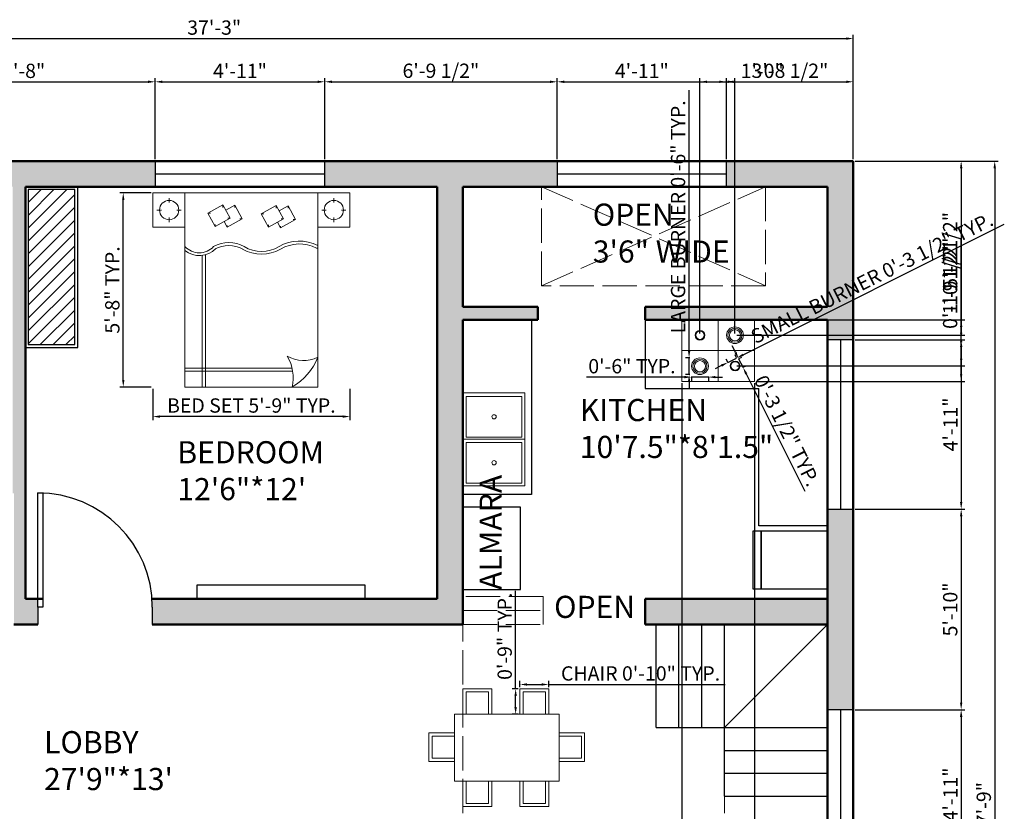
# Model space of a CAD drawing. Units: inches. Extents: x 876 to 1414, y 2665 to 3216.
# Tile 4 of 4: x 1070 to 1414, y 2939 to 3216. Entities that reach past the tile are written whole.
import ezdxf

# ---------------------------------------------------------------- set-up
doc = ezdxf.new("R2010")
doc.units = ezdxf.units.IN
doc.linetypes.add('ACAD_ISO02W100', pattern=[15, 12, -3])
for name, color, linetype, lineweight in [('A-ANNO-DIMS', 2, 'Continuous', 18), ('A-ANNO-TEXT', 7, 'Continuous', 25), ('A-AREA-IDEN', 7, 'Continuous', 25), ('A-EQPM', 9, 'Continuous', 18), ('A-FLOR-CASE', 8, 'Continuous', 25), ('A-FLOR-CASE-PATT', 252, 'Continuous', 13), ('A-FLOR-FIXT', 9, 'Continuous', 18), ('A-FLOR-STRS', 150, 'Continuous', 25), ('A-FLOR-STRS-OVHD', 150, 'ACAD_ISO02W100', 18), ('A-OPEN-OVHD', 210, 'ACAD_ISO02W100', 18), ('A-WALL-PATT', 252, 'Continuous', 13), ('DOOR', 52, 'Continuous', 25), ('FUR', 8, 'Continuous', 18), ('KIT', 40, 'Continuous', 25), ('WALL', 7, 'Continuous', 50), ('WIND', 130, 'Continuous', 25)]:
    doc.layers.add(name, color=color, linetype=linetype, lineweight=lineweight)
doc.styles.get("Standard").update_dxf_attribs({"font": 'arial.ttf'})
doc.dimstyles.new('ISO-25', dxfattribs={"dimtxt": 5, "dimasz": 2.5, "dimexe": 1.25, "dimexo": 0.625, "dimtad": 1, "dimdec": 0, "dimlunit": 4, "dimtxsty": 'Standard', "dimcen": 2.5, "dimadec": 0, "dimazin": 0, "dimtfac": 1, "dimtdec": 0, "dimtmove": 0, "dimatfit": 3, "dimfxl": 1, "dimarcsym": 0})

# ---------------------------------------------------------------- blocks, each defined once
blk = doc.blocks.new('*U2')
for p, q in [((0, 0), (0, -6)), ((40, 0), (40, -6))]:
    blk.add_line(p, q)
blk.add_lwpolyline([(0, 0), (0, 40), (1.75, 40), (1.75, 0)], close=True)
blk.add_arc((0, 0), 40, 0, 90)
blk = doc.blocks.new('*D7')
at = {"layer": 'A-ANNO-DIMS', "color": 0, "lineweight": -2, "transparency": 16777216}
for p, q in [((914.52, 3167.07), (914.52, 3210.51)), ((917.02, 3209.26), (1359.02, 3209.26)), ((1361.52, 3167.07), (1361.52, 3210.51))]:
    blk.add_line(p, q, dxfattribs=at)
at = {"layer": 'A-ANNO-DIMS', "color": 0, "lineweight": 100, "transparency": 16777216}
for points in [[(917.02, 3209.68), (917.02, 3208.84), (914.52, 3209.26)], [(1359.02, 3209.68), (1359.02, 3208.84), (1361.52, 3209.26)]]:
    blk.add_solid(points, dxfattribs=at)
at = {"layer": 'Defpoints', "color": 0, "lineweight": 100, "transparency": 16777216}
for p in [(1361.52, 3209.26), (914.52, 3166.44), (1361.52, 3166.44)]:
    blk.add_point(p, dxfattribs=at)
at = {"layer": 'A-ANNO-DIMS', "color": 0, "transparency": 16777216, "insert": (1138.02, 3212.44), "char_height": 5, "attachment_point": 5}
blk.add_mtext('37\'-3"', dxfattribs=at)
blk = doc.blocks.new('*D8')
at = {"layer": 'A-ANNO-DIMS', "color": 0, "lineweight": -2, "transparency": 16777216}
for p, q in [((1362.14, 3166.44), (1412.22, 3166.44)), ((1410.97, 3163.94), (1410.97, 2715.94)), ((1362.14, 2713.44), (1412.22, 2713.44))]:
    blk.add_line(p, q, dxfattribs=at)
at = {"layer": 'A-ANNO-DIMS', "color": 0, "lineweight": 100, "transparency": 16777216}
for points in [[(1410.55, 3163.94), (1411.38, 3163.94), (1410.97, 3166.44)], [(1410.55, 2715.94), (1411.38, 2715.94), (1410.97, 2713.44)]]:
    blk.add_solid(points, dxfattribs=at)
at = {"layer": 'Defpoints', "color": 0, "lineweight": 100, "transparency": 16777216}
for p in [(1361.52, 3166.44), (1361.52, 2713.44), (1410.97, 2713.44)]:
    blk.add_point(p, dxfattribs=at)
at = {"layer": 'A-ANNO-DIMS', "color": 0, "transparency": 16777216, "insert": (1407.79, 2939.94), "char_height": 5, "attachment_point": 5, "rotation": 90}
blk.add_mtext('37\'-9"', dxfattribs=at)
blk = doc.blocks.new('BED-DOUBLE-NIGHTSTANDS')
for p, q in [((61.86, 66.59), (61.86, 67.46)), ((61.86, 66.59), (61.86, 65.9)), ((58.48, 63.21), (57.64, 63.21)), ((58.48, 63.21), (59.22, 63.21)), ((65.24, 63.21), (64.53, 63.21)), ((65.24, 63.21), (66.05, 63.21)), ((61.86, 59.83), (61.86, 60.56)), ((61.86, 59.83), (61.86, 59.02)), ((5.55, 20.02), (5.55, 57.68)), ((5.55, 20.02), (5.55, 57.68)), ((6.55, 20.22), (6.55, 57.68)), ((0, 51.64), (45.97, 51.64)), ((0, 50.51), (45.97, 50.51)), ((45.97, 50.51), (46.2, 50.51)), ((60.79, 49.72), (60.79, 48.79)), ((56.06, 47.08), (56.85, 47.08)), ((55.87, 42.88), (56.5, 42.88)), ((58.98, 41.84), (58.98, 42.69)), ((63.72, 44.49), (62.78, 44.49)), ((58.79, 37.65), (58.79, 38.47)), ((63.53, 40.29), (62.71, 40.29)), ((60.58, 31.07), (60.58, 30.14)), ((55.85, 28.43), (56.64, 28.43)), ((55.66, 24.23), (56.28, 24.23)), ((63.5, 25.84), (62.57, 25.84)), ((58.77, 23.19), (58.77, 24.04)), ((63.31, 21.64), (62.5, 21.64)), ((58.58, 19), (58.58, 19.82)), ((48.54, 11.7), (48.54, 11.24)), ((61.86, 9), (61.86, 9.87)), ((61.86, 9), (61.86, 8.3)), ((58.48, 5.62), (57.64, 5.62)), ((58.48, 5.62), (59.22, 5.62)), ((65.24, 5.62), (64.53, 5.62)), ((65.24, 5.62), (66.05, 5.62)), ((61.86, 2.24), (61.86, 2.97)), ((61.86, 2.24), (61.86, 1.43))]:
    blk.add_line(p, q)
for points in [[(67.84, 57.68), (55.89, 57.68), (55.89, 68.92), (67.84, 68.92)], [(67.84, 57.68), (0, 57.68), (0, 11.24), (67.84, 11.24)], [(60.79, 49.72), (63.72, 44.49), (58.98, 41.84), (56.06, 47.08)], [(60.58, 31.07), (63.5, 25.84), (58.77, 23.19), (55.85, 28.43)], [(67.84, 0), (55.89, 0), (55.89, 11.24), (67.84, 11.24)]]:
    blk.add_lwpolyline(points, close=True)
for points in [[(61.78, 43.41), (63.53, 40.29), (58.79, 37.65), (55.87, 42.88), (57.8, 43.96)], [(61.57, 24.76), (63.31, 21.64), (58.58, 19), (55.66, 24.23), (57.59, 25.31)]]:
    blk.add_lwpolyline(points)
for centre in [(61.86, 63.21), (61.86, 5.62)]:
    blk.add_circle(centre, 3.38)
for centre, radius, start, end in [((53.77, 52.67), 7.86, 140.4162, 226.8897), ((53.77, 52.67), 6.86, 133.1103, 226.8897), ((39.66, 42.33), 9.82, 330.4833, 29.5167), ((39.66, 42.33), 10.82, 330.4833, 29.5167), ((59.48, 30.89), 13.07, 149.6109, 210.3891), ((59.48, 30.89), 12.07, 149.6109, 210.3891), ((37, 17.69), 13, 332.5506, 30.4499), ((37, 17.69), 14, 332.5506, 30.4499), ((3.14, 34.99), 15.16, 258.0495, 300.2653), ((20.79, 16.21), 11.51, 150.3891, 205.6064), ((18.12, 30.76), 20.99, 210.3296, 248.4534)]:
    blk.add_arc(centre, radius, start, end)
blk = doc.blocks.new('CHAIR-DINING')
for p, q in [((0, 0), (0, 8.9)), ((0, 8.9), (10.06, 8.9)), ((10.06, 8.9), (10.06, 0))]:
    blk.add_line(p, q)
blk.add_lwpolyline([(1.15, 0), (8.89, 0), (8.89, 7.82), (1.15, 7.82)], close=True)
blk = doc.blocks.new('HOB-BURNER-SMALL')
for radius in [1.71, 1.71, 1.46]:
    blk.add_circle((1.71, 1.71), radius)
blk = doc.blocks.new('HOB-BURNER-LARGE')
for radius in [2.93, 2.44, 1.96]:
    blk.add_circle((2.93, 2.93), radius)
blk = doc.blocks.new('*D14')
at = {"layer": 'A-ANNO-DIMS', "color": 0, "lineweight": -2, "transparency": 16777216}
for p, q in [((1244.94, 2982.58), (1244.94, 2984.71)), ((1247.44, 2983.46), (1252.5, 2983.46)), ((1255, 2982.58), (1255, 2984.71)), ((1255, 2983.46), (1316.73, 2983.46))]:
    blk.add_line(p, q, dxfattribs=at)
at = {"layer": 'A-ANNO-DIMS', "color": 0, "lineweight": 100, "transparency": 16777216}
for points in [[(1247.44, 2983.88), (1247.44, 2983.05), (1244.94, 2983.46)], [(1252.5, 2983.88), (1252.5, 2983.05), (1255, 2983.46)]]:
    blk.add_solid(points, dxfattribs=at)
at = {"layer": 'Defpoints', "color": 0, "lineweight": 100, "transparency": 16777216}
for p in [(1244.94, 2981.95), (1255, 2983.46), (1255, 2981.95)]:
    blk.add_point(p, dxfattribs=at)
at = {"layer": 'A-ANNO-DIMS', "color": 0, "transparency": 16777216, "insert": (1287.11, 2986.67), "char_height": 5, "attachment_point": 5}
blk.add_mtext('CHAIR 0\'-10" TYP.', dxfattribs=at)
blk = doc.blocks.new('*D15')
at = {"layer": 'A-ANNO-DIMS', "color": 0, "lineweight": -2, "transparency": 16777216}
for p, q in [((1243.43, 2981.95), (1243.43, 3016.18)), ((1244.31, 2981.95), (1242.18, 2981.95)), ((1243.43, 2975.56), (1243.43, 2979.45)), ((1244.31, 2973.06), (1242.18, 2973.06))]:
    blk.add_line(p, q, dxfattribs=at)
at = {"layer": 'A-ANNO-DIMS', "color": 0, "lineweight": 100, "transparency": 16777216}
for points in [[(1243.01, 2979.45), (1243.85, 2979.45), (1243.43, 2981.95)], [(1243.01, 2975.56), (1243.85, 2975.56), (1243.43, 2973.06)]]:
    blk.add_solid(points, dxfattribs=at)
at = {"layer": 'Defpoints', "color": 0, "lineweight": 100, "transparency": 16777216}
for p in [(1243.43, 2981.95), (1244.94, 2981.95), (1244.94, 2973.06)]:
    blk.add_point(p, dxfattribs=at)
at = {"layer": 'A-ANNO-DIMS', "color": 0, "transparency": 16777216, "insert": (1240.25, 3000.32), "char_height": 5, "attachment_point": 5, "rotation": 90}
blk.add_mtext('0\'-9" TYP.', dxfattribs=at)
blk = doc.blocks.new('*D16')
at = {"layer": 'A-ANNO-DIMS', "color": 0, "lineweight": -2, "transparency": 16777216}
for p, q in [((1116.56, 3086.83), (1116.56, 3075.87)), ((1185.48, 3086.83), (1185.48, 3075.87)), ((1182.98, 3077.12), (1119.06, 3077.12))]:
    blk.add_line(p, q, dxfattribs=at)
at = {"layer": 'A-ANNO-DIMS', "color": 0, "lineweight": 100, "transparency": 16777216}
for points in [[(1119.06, 3077.53), (1119.06, 3076.7), (1116.56, 3077.12)], [(1182.98, 3077.53), (1182.98, 3076.7), (1185.48, 3077.12)]]:
    blk.add_solid(points, dxfattribs=at)
at = {"layer": 'Defpoints', "color": 0, "lineweight": 100, "transparency": 16777216}
for p in [(1116.56, 3087.45), (1185.48, 3087.45), (1116.56, 3077.12)]:
    blk.add_point(p, dxfattribs=at)
at = {"layer": 'A-ANNO-DIMS', "color": 0, "transparency": 16777216, "insert": (1151.02, 3080.33), "char_height": 5, "attachment_point": 5}
blk.add_mtext('BED SET 5\'-9" TYP.', dxfattribs=at)
blk = doc.blocks.new('*D17')
at = {"layer": 'A-ANNO-DIMS', "color": 0, "lineweight": -2, "transparency": 16777216}
for p, q in [((1115.94, 3155.29), (1104.97, 3155.29)), ((1106.22, 3089.95), (1106.22, 3152.79)), ((1115.94, 3087.45), (1104.97, 3087.45))]:
    blk.add_line(p, q, dxfattribs=at)
at = {"layer": 'A-ANNO-DIMS', "color": 0, "lineweight": 100, "transparency": 16777216}
for points in [[(1105.81, 3152.79), (1106.64, 3152.79), (1106.22, 3155.29)], [(1105.81, 3089.95), (1106.64, 3089.95), (1106.22, 3087.45)]]:
    blk.add_solid(points, dxfattribs=at)
at = {"layer": 'Defpoints', "color": 0, "lineweight": 100, "transparency": 16777216}
for p in [(1106.22, 3155.29), (1116.56, 3155.29), (1116.56, 3087.45)]:
    blk.add_point(p, dxfattribs=at)
at = {"layer": 'A-ANNO-DIMS', "color": 0, "transparency": 16777216, "insert": (1103.05, 3121.37), "char_height": 5, "attachment_point": 5, "rotation": 90}
blk.add_mtext('5\'-8" TYP.', dxfattribs=at)
blk = doc.blocks.new('*D20')
at = {"layer": 'A-ANNO-DIMS', "color": 0, "lineweight": -2, "transparency": 16777216}
for p, q in [((1322.96, 3098.7), (1414.31, 3144.37)), ((1317.62, 3096.15), (1317.11, 3097.17)), ((1317.67, 3096.05), (1320.72, 3097.58)), ((1320.67, 3097.68), (1320.16, 3098.7)), ((1315.43, 3094.93), (1313.19, 3093.82))]:
    blk.add_line(p, q, dxfattribs=at)
at = {"layer": 'A-ANNO-DIMS', "color": 0, "lineweight": 100, "transparency": 16777216}
for points in [[(1322.77, 3099.07), (1323.15, 3098.33), (1320.72, 3097.58)], [(1315.24, 3095.31), (1315.62, 3094.56), (1317.67, 3096.05)]]:
    blk.add_solid(points, dxfattribs=at)
at = {"layer": 'Defpoints', "color": 0, "lineweight": 100, "transparency": 16777216}
for p in [(1317.9, 3095.59), (1320.72, 3097.58), (1320.95, 3097.12)]:
    blk.add_point(p, dxfattribs=at)
at = {"layer": 'A-ANNO-DIMS', "color": 0, "transparency": 16777216, "insert": (1368.32, 3124.97), "char_height": 5, "attachment_point": 5, "rotation": 26.5651}
blk.add_mtext('SMALL BURNER 0\'-3 1/2" TYP.', dxfattribs=at)
blk = doc.blocks.new('*D21')
at = {"layer": 'A-ANNO-DIMS', "color": 0, "lineweight": -2, "transparency": 16777216}
for p, q in [((1320.29, 3099.59), (1319.18, 3101.82)), ((1321.41, 3097.35), (1322.94, 3094.29)), ((1321.51, 3097.4), (1322.53, 3097.91)), ((1323.04, 3094.34), (1324.06, 3094.85)), ((1324.06, 3092.06), (1344.57, 3051.02))]:
    blk.add_line(p, q, dxfattribs=at)
at = {"layer": 'A-ANNO-DIMS', "color": 0, "lineweight": 100, "transparency": 16777216}
for points in [[(1320.67, 3099.77), (1319.92, 3099.4), (1321.41, 3097.35)], [(1324.43, 3092.24), (1323.68, 3091.87), (1322.94, 3094.29)]]:
    blk.add_solid(points, dxfattribs=at)
at = {"layer": 'Defpoints', "color": 0, "lineweight": 100, "transparency": 16777216}
for p in [(1320.95, 3097.12), (1322.48, 3094.06), (1322.94, 3094.29)]:
    blk.add_point(p, dxfattribs=at)
at = {"layer": 'A-ANNO-DIMS', "color": 0, "transparency": 16777216, "insert": (1337.75, 3071.86), "char_height": 5, "attachment_point": 5, "rotation": 296.5651}
blk.add_mtext('0\'-3 1/2" TYP.', dxfattribs=at)
blk = doc.blocks.new('*D22')
at = {"layer": 'A-ANNO-DIMS', "color": 0, "lineweight": -2, "transparency": 16777216}
for p, q in [((1304.09, 3100.14), (1304.09, 3191.2)), ((1304.34, 3097.64), (1302.84, 3097.64)), ((1304.09, 3091.78), (1304.09, 3097.64)), ((1304.34, 3091.78), (1302.84, 3091.78)), ((1304.09, 3089.28), (1304.09, 3086.78))]:
    blk.add_line(p, q, dxfattribs=at)
at = {"layer": 'A-ANNO-DIMS', "color": 0, "lineweight": 100, "transparency": 16777216}
for points in [[(1303.67, 3100.14), (1304.51, 3100.14), (1304.09, 3097.64)], [(1303.67, 3089.28), (1304.51, 3089.28), (1304.09, 3091.78)]]:
    blk.add_solid(points, dxfattribs=at)
at = {"layer": 'Defpoints', "color": 0, "lineweight": 100, "transparency": 16777216}
for p in [(1304.09, 3097.64), (1304.97, 3097.64), (1304.97, 3091.78)]:
    blk.add_point(p, dxfattribs=at)
at = {"layer": 'A-ANNO-DIMS', "color": 0, "transparency": 16777216, "insert": (1300.88, 3146.92), "char_height": 5, "attachment_point": 5, "rotation": 90}
blk.add_mtext('LARGE BURNER 0\'-6" TYP.', dxfattribs=at)
blk = doc.blocks.new('*D23')
at = {"layer": 'A-ANNO-DIMS', "color": 0, "lineweight": -2, "transparency": 16777216}
for p, q in [((1302.47, 3090.91), (1268.24, 3090.91)), ((1304.97, 3091.16), (1304.97, 3089.66)), ((1310.82, 3090.91), (1304.97, 3090.91)), ((1310.82, 3091.16), (1310.82, 3089.66)), ((1313.32, 3090.91), (1315.82, 3090.91))]:
    blk.add_line(p, q, dxfattribs=at)
at = {"layer": 'A-ANNO-DIMS', "color": 0, "lineweight": 100, "transparency": 16777216}
for points in [[(1302.47, 3091.32), (1302.47, 3090.49), (1304.97, 3090.91)], [(1313.32, 3091.32), (1313.32, 3090.49), (1310.82, 3090.91)]]:
    blk.add_solid(points, dxfattribs=at)
at = {"layer": 'Defpoints', "color": 0, "lineweight": 100, "transparency": 16777216}
for p in [(1304.97, 3091.78), (1304.97, 3090.91), (1310.82, 3091.78)]:
    blk.add_point(p, dxfattribs=at)
at = {"layer": 'A-ANNO-DIMS', "color": 0, "transparency": 16777216, "insert": (1284.1, 3094.08), "char_height": 5, "attachment_point": 5}
blk.add_mtext('0\'-6" TYP.', dxfattribs=at)
blk = doc.blocks.new('*D24')
at = {"layer": 'A-ANNO-DIMS', "color": 0, "lineweight": -2, "transparency": 16777216}
for p, q in [((1301.58, 3088.78), (1301.58, 2682.56)), ((1326.96, 3088.78), (1326.96, 2682.56)), ((1304.08, 2683.81), (1324.46, 2683.81)), ((1326.96, 2683.81), (1355.74, 2683.81))]:
    blk.add_line(p, q, dxfattribs=at)
at = {"layer": 'A-ANNO-DIMS', "color": 0, "lineweight": 100, "transparency": 16777216}
for points in [[(1304.08, 2684.22), (1304.08, 2683.39), (1301.58, 2683.81)], [(1324.46, 2684.22), (1324.46, 2683.39), (1326.96, 2683.81)]]:
    blk.add_solid(points, dxfattribs=at)
at = {"layer": 'Defpoints', "color": 0, "lineweight": 100, "transparency": 16777216}
for p in [(1301.58, 3089.41), (1326.96, 3089.41), (1326.96, 2683.81)]:
    blk.add_point(p, dxfattribs=at)
at = {"layer": 'A-ANNO-DIMS', "color": 0, "transparency": 16777216, "insert": (1342.6, 2687.02), "char_height": 5, "attachment_point": 5}
blk.add_mtext('2\'-1 1/2"', dxfattribs=at)
blk = doc.blocks.new('*D25')
at = {"layer": 'A-ANNO-DIMS', "color": 0, "lineweight": -2, "transparency": 16777216}
for p, q in [((1399.23, 3110.94), (1399.23, 3139.16)), ((1327.59, 3110.94), (1400.48, 3110.94)), ((1399.23, 3091.91), (1399.23, 3108.44)), ((1327.59, 3089.41), (1400.48, 3089.41))]:
    blk.add_line(p, q, dxfattribs=at)
at = {"layer": 'A-ANNO-DIMS', "color": 0, "lineweight": 100, "transparency": 16777216}
for points in [[(1398.82, 3108.44), (1399.65, 3108.44), (1399.23, 3110.94)], [(1398.82, 3091.91), (1399.65, 3091.91), (1399.23, 3089.41)]]:
    blk.add_solid(points, dxfattribs=at)
at = {"layer": 'Defpoints', "color": 0, "lineweight": 100, "transparency": 16777216}
for p in [(1326.96, 3110.94), (1399.23, 3110.94), (1326.96, 3089.41)]:
    blk.add_point(p, dxfattribs=at)
at = {"layer": 'A-ANNO-DIMS', "color": 0, "transparency": 16777216, "insert": (1396.02, 3126.3), "char_height": 5, "attachment_point": 5, "rotation": 90}
blk.add_mtext('1\'-9 1/2"', dxfattribs=at)
blk = doc.blocks.new('*D26')
at = {"layer": 'A-ANNO-DIMS', "color": 0, "lineweight": -2, "transparency": 16777216}
for p, q in [((1307.9, 3106.17), (1307.9, 3195.39)), ((1320.13, 3106.16), (1320.13, 3195.39)), ((1310.4, 3194.14), (1317.63, 3194.14)), ((1320.13, 3194.14), (1336.7, 3194.14))]:
    blk.add_line(p, q, dxfattribs=at)
at = {"layer": 'A-ANNO-DIMS', "color": 0, "lineweight": 100, "transparency": 16777216}
for points in [[(1310.4, 3194.56), (1310.4, 3193.72), (1307.9, 3194.14)], [(1317.63, 3194.56), (1317.63, 3193.72), (1320.13, 3194.14)]]:
    blk.add_solid(points, dxfattribs=at)
at = {"layer": 'Defpoints', "color": 0, "lineweight": 100, "transparency": 16777216}
for p in [(1320.13, 3194.14), (1307.9, 3105.55), (1320.13, 3105.54)]:
    blk.add_point(p, dxfattribs=at)
at = {"layer": 'A-ANNO-DIMS', "color": 0, "transparency": 16777216, "insert": (1329.66, 3197.32), "char_height": 5, "attachment_point": 5}
blk.add_mtext('1\'-0"', dxfattribs=at)
blk = doc.blocks.new('*D27')
at = {"layer": 'A-ANNO-DIMS', "color": 0, "lineweight": -2, "transparency": 16777216}
for p, q in [((1399.23, 3105.54), (1399.23, 3138.11)), ((1320.75, 3105.54), (1400.48, 3105.54)), ((1399.23, 3097.33), (1399.23, 3103.04)), ((1320.81, 3094.83), (1400.48, 3094.83))]:
    blk.add_line(p, q, dxfattribs=at)
at = {"layer": 'A-ANNO-DIMS', "color": 0, "lineweight": 100, "transparency": 16777216}
for points in [[(1398.82, 3103.04), (1399.65, 3103.04), (1399.23, 3105.54)], [(1398.82, 3097.33), (1399.65, 3097.33), (1399.23, 3094.83)]]:
    blk.add_solid(points, dxfattribs=at)
at = {"layer": 'Defpoints', "color": 0, "lineweight": 100, "transparency": 16777216}
for p in [(1320.13, 3105.54), (1399.23, 3105.54), (1320.19, 3094.83)]:
    blk.add_point(p, dxfattribs=at)
at = {"layer": 'A-ANNO-DIMS', "color": 0, "transparency": 16777216, "insert": (1396.02, 3123.07), "char_height": 5, "attachment_point": 5, "rotation": 90}
blk.add_mtext('0\'-10 1/2"', dxfattribs=at)
blk = doc.blocks.new('*D36')
at = {"layer": 'A-ANNO-DIMS', "color": 0, "lineweight": -2, "transparency": 16777216}
for p, q in [((1025.39, 3167.07), (1025.39, 3195.39)), ((1117.41, 3167.07), (1117.41, 3195.39)), ((1027.89, 3194.14), (1114.91, 3194.14))]:
    blk.add_line(p, q, dxfattribs=at)
at = {"layer": 'A-ANNO-DIMS', "color": 0, "lineweight": 100, "transparency": 16777216}
for points in [[(1027.89, 3194.56), (1027.89, 3193.72), (1025.39, 3194.14)], [(1114.91, 3194.56), (1114.91, 3193.72), (1117.41, 3194.14)]]:
    blk.add_solid(points, dxfattribs=at)
at = {"layer": 'Defpoints', "color": 0, "lineweight": 100, "transparency": 16777216}
for p in [(1117.41, 3194.14), (1025.39, 3166.44), (1117.41, 3166.44)]:
    blk.add_point(p, dxfattribs=at)
at = {"layer": 'A-ANNO-DIMS', "color": 0, "transparency": 16777216, "insert": (1071.4, 3197.32), "char_height": 5, "attachment_point": 5}
blk.add_mtext('7\'-8"', dxfattribs=at)
blk = doc.blocks.new('*D37')
at = {"layer": 'A-ANNO-DIMS', "color": 0, "lineweight": -2, "transparency": 16777216}
for p, q in [((1117.41, 3167.07), (1117.41, 3195.39)), ((1176.66, 3167.07), (1176.66, 3195.39)), ((1119.91, 3194.14), (1174.16, 3194.14))]:
    blk.add_line(p, q, dxfattribs=at)
at = {"layer": 'A-ANNO-DIMS', "color": 0, "lineweight": 100, "transparency": 16777216}
for points in [[(1119.91, 3194.56), (1119.91, 3193.72), (1117.41, 3194.14)], [(1174.16, 3194.56), (1174.16, 3193.72), (1176.66, 3194.14)]]:
    blk.add_solid(points, dxfattribs=at)
at = {"layer": 'Defpoints', "color": 0, "lineweight": 100, "transparency": 16777216}
for p in [(1176.66, 3194.14), (1117.41, 3166.44), (1176.66, 3166.44)]:
    blk.add_point(p, dxfattribs=at)
at = {"layer": 'A-ANNO-DIMS', "color": 0, "transparency": 16777216, "insert": (1147.04, 3197.28), "char_height": 5, "attachment_point": 5}
blk.add_mtext('4\'-11"', dxfattribs=at)
blk = doc.blocks.new('*D38')
at = {"layer": 'A-ANNO-DIMS', "color": 0, "lineweight": -2, "transparency": 16777216}
for p, q in [((1176.66, 3167.07), (1176.66, 3195.39)), ((1257.93, 3167.07), (1257.93, 3195.39)), ((1179.16, 3194.14), (1255.43, 3194.14))]:
    blk.add_line(p, q, dxfattribs=at)
at = {"layer": 'A-ANNO-DIMS', "color": 0, "lineweight": 100, "transparency": 16777216}
for points in [[(1179.16, 3194.56), (1179.16, 3193.72), (1176.66, 3194.14)], [(1255.43, 3194.56), (1255.43, 3193.72), (1257.93, 3194.14)]]:
    blk.add_solid(points, dxfattribs=at)
at = {"layer": 'Defpoints', "color": 0, "lineweight": 100, "transparency": 16777216}
for p in [(1257.93, 3194.14), (1176.66, 3166.44), (1257.93, 3166.44)]:
    blk.add_point(p, dxfattribs=at)
at = {"layer": 'A-ANNO-DIMS', "color": 0, "transparency": 16777216, "insert": (1217.3, 3197.35), "char_height": 5, "attachment_point": 5}
blk.add_mtext('6\'-9 1/2"', dxfattribs=at)
blk = doc.blocks.new('*D39')
at = {"layer": 'A-ANNO-DIMS', "color": 0, "lineweight": -2, "transparency": 16777216}
for p, q in [((1257.93, 3167.07), (1257.93, 3195.39)), ((1317.18, 3167.07), (1317.18, 3195.39)), ((1260.43, 3194.14), (1314.68, 3194.14))]:
    blk.add_line(p, q, dxfattribs=at)
at = {"layer": 'A-ANNO-DIMS', "color": 0, "lineweight": 100, "transparency": 16777216}
for points in [[(1260.43, 3194.56), (1260.43, 3193.72), (1257.93, 3194.14)], [(1314.68, 3194.56), (1314.68, 3193.72), (1317.18, 3194.14)]]:
    blk.add_solid(points, dxfattribs=at)
at = {"layer": 'Defpoints', "color": 0, "lineweight": 100, "transparency": 16777216}
for p in [(1317.18, 3194.14), (1257.93, 3166.44), (1317.18, 3166.44)]:
    blk.add_point(p, dxfattribs=at)
at = {"layer": 'A-ANNO-DIMS', "color": 0, "transparency": 16777216, "insert": (1287.56, 3197.28), "char_height": 5, "attachment_point": 5}
blk.add_mtext('4\'-11"', dxfattribs=at)
blk = doc.blocks.new('*D40')
at = {"layer": 'A-ANNO-DIMS', "color": 0, "lineweight": -2, "transparency": 16777216}
for p, q in [((1317.18, 3167.07), (1317.18, 3195.39)), ((1361.52, 3167.07), (1361.52, 3195.39)), ((1319.68, 3194.14), (1359.02, 3194.14))]:
    blk.add_line(p, q, dxfattribs=at)
at = {"layer": 'A-ANNO-DIMS', "color": 0, "lineweight": 100, "transparency": 16777216}
for points in [[(1319.68, 3194.56), (1319.68, 3193.72), (1317.18, 3194.14)], [(1359.02, 3194.56), (1359.02, 3193.72), (1361.52, 3194.14)]]:
    blk.add_solid(points, dxfattribs=at)
at = {"layer": 'Defpoints', "color": 0, "lineweight": 100, "transparency": 16777216}
for p in [(1361.52, 3194.14), (1317.18, 3166.44), (1361.52, 3166.44)]:
    blk.add_point(p, dxfattribs=at)
at = {"layer": 'A-ANNO-DIMS', "color": 0, "transparency": 16777216, "insert": (1339.35, 3197.35), "char_height": 5, "attachment_point": 5}
blk.add_mtext('3\'-8 1/2"', dxfattribs=at)
blk = doc.blocks.new('*D54')
at = {"layer": 'A-ANNO-DIMS', "color": 0, "lineweight": -2, "transparency": 16777216}
for p, q in [((1362.14, 3166.44), (1400.48, 3166.44)), ((1399.23, 3163.94), (1399.23, 3106.48)), ((1362.14, 3103.98), (1400.48, 3103.98))]:
    blk.add_line(p, q, dxfattribs=at)
at = {"layer": 'A-ANNO-DIMS', "color": 0, "lineweight": 100, "transparency": 16777216}
for points in [[(1398.82, 3163.94), (1399.65, 3163.94), (1399.23, 3166.44)], [(1398.82, 3106.48), (1399.65, 3106.48), (1399.23, 3103.98)]]:
    blk.add_solid(points, dxfattribs=at)
at = {"layer": 'Defpoints', "color": 0, "lineweight": 100, "transparency": 16777216}
for p in [(1361.52, 3166.44), (1361.52, 3103.98), (1399.23, 3103.98)]:
    blk.add_point(p, dxfattribs=at)
at = {"layer": 'A-ANNO-DIMS', "color": 0, "transparency": 16777216, "insert": (1396.02, 3135.21), "char_height": 5, "attachment_point": 5, "rotation": 90}
blk.add_mtext('5\'-2 1/2"', dxfattribs=at)
blk = doc.blocks.new('*D55')
at = {"layer": 'A-ANNO-DIMS', "color": 0, "lineweight": -2, "transparency": 16777216}
for p, q in [((1362.14, 3103.98), (1400.48, 3103.98)), ((1399.23, 3101.48), (1399.23, 3047.23)), ((1362.14, 3044.73), (1400.48, 3044.73))]:
    blk.add_line(p, q, dxfattribs=at)
at = {"layer": 'A-ANNO-DIMS', "color": 0, "lineweight": 100, "transparency": 16777216}
for points in [[(1398.82, 3101.48), (1399.65, 3101.48), (1399.23, 3103.98)], [(1398.82, 3047.23), (1399.65, 3047.23), (1399.23, 3044.73)]]:
    blk.add_solid(points, dxfattribs=at)
at = {"layer": 'Defpoints', "color": 0, "lineweight": 100, "transparency": 16777216}
for p in [(1361.52, 3103.98), (1361.52, 3044.73), (1399.23, 3044.73)]:
    blk.add_point(p, dxfattribs=at)
at = {"layer": 'A-ANNO-DIMS', "color": 0, "transparency": 16777216, "insert": (1396.1, 3074.36), "char_height": 5, "attachment_point": 5, "rotation": 90}
blk.add_mtext('4\'-11"', dxfattribs=at)
blk = doc.blocks.new('*D56')
at = {"layer": 'A-ANNO-DIMS', "color": 0, "lineweight": -2, "transparency": 16777216}
for p, q in [((1362.14, 3044.73), (1400.48, 3044.73)), ((1399.23, 3042.23), (1399.23, 2977.15)), ((1362.14, 2974.65), (1400.48, 2974.65))]:
    blk.add_line(p, q, dxfattribs=at)
at = {"layer": 'A-ANNO-DIMS', "color": 0, "lineweight": 100, "transparency": 16777216}
for points in [[(1398.82, 3042.23), (1399.65, 3042.23), (1399.23, 3044.73)], [(1398.82, 2977.15), (1399.65, 2977.15), (1399.23, 2974.65)]]:
    blk.add_solid(points, dxfattribs=at)
at = {"layer": 'Defpoints', "color": 0, "lineweight": 100, "transparency": 16777216}
for p in [(1361.52, 3044.73), (1361.52, 2974.65), (1399.23, 2974.65)]:
    blk.add_point(p, dxfattribs=at)
at = {"layer": 'A-ANNO-DIMS', "color": 0, "transparency": 16777216, "insert": (1396.05, 3009.69), "char_height": 5, "attachment_point": 5, "rotation": 90}
blk.add_mtext('5\'-10"', dxfattribs=at)
blk = doc.blocks.new('*D57')
at = {"layer": 'A-ANNO-DIMS', "color": 0, "lineweight": -2, "transparency": 16777216}
for p, q in [((1362.14, 2974.65), (1400.48, 2974.65)), ((1399.23, 2972.15), (1399.23, 2917.9)), ((1362.14, 2915.4), (1400.48, 2915.4))]:
    blk.add_line(p, q, dxfattribs=at)
at = {"layer": 'A-ANNO-DIMS', "color": 0, "lineweight": 100, "transparency": 16777216}
for points in [[(1398.82, 2972.15), (1399.65, 2972.15), (1399.23, 2974.65)], [(1398.82, 2917.9), (1399.65, 2917.9), (1399.23, 2915.4)]]:
    blk.add_solid(points, dxfattribs=at)
at = {"layer": 'Defpoints', "color": 0, "lineweight": 100, "transparency": 16777216}
for p in [(1361.52, 2974.65), (1361.52, 2915.4), (1399.23, 2915.4)]:
    blk.add_point(p, dxfattribs=at)
at = {"layer": 'A-ANNO-DIMS', "color": 0, "transparency": 16777216, "insert": (1396.1, 2945.02), "char_height": 5, "attachment_point": 5, "rotation": 90}
blk.add_mtext('4\'-11"', dxfattribs=at)

msp = doc.modelspace()

# ---------------------------------------------------------------- hatches: boundary and pattern name
at = {"layer": 'A-FLOR-CASE-PATT'}
h = msp.add_hatch(dxfattribs=at)
h.set_pattern_fill('ANSI31', color=256)
h.paths.add_polyline_path([(1089.31, 3156.44), (1073.02, 3156.44), (1073.02, 3102.26), (1089.31, 3102.26)])
at = {"layer": 'A-WALL-PATT'}
h = msp.add_hatch(color=256, dxfattribs=at)
h.dxf.hatch_style = 1
h.paths.add_polyline_path([(966.14, 3166.44), (914.52, 3166.44), (914.52, 3077.43), (923.52, 3077.43), (923.52, 3157.44), (966.14, 3157.44)])
h.paths.add_polyline_path([(1117.41, 3166.44), (1072.02, 3166.44), (1025.39, 3166.44), (1025.39, 3157.44), (1067.52, 3157.44), (1067.52, 3050.33), (1068, 3050.33), (1068, 3010.33), (1068, 3004.44), (1072.02, 3004.44), (1076.39, 3004.44), (1076.39, 3010.44), (1076.39, 3013.44), (1072.02, 3013.44), (1072.02, 3157.44), (1090.31, 3157.44), (1117.41, 3157.44)])
h.paths.add_polyline_path([(1257.93, 3166.44), (1225.02, 3166.44), (1176.66, 3166.44), (1176.66, 3157.44), (1216.02, 3157.44), (1216.02, 3013.44), (1116.28, 3013.44, -0.01877), (1116.39, 3010.44), (1116.39, 3004.44), (1225.02, 3004.44), (1225.02, 3014.27), (1225.02, 3110.94), (1249.02, 3110.94), (1251.21, 3110.94), (1251.21, 3115.44), (1225.02, 3115.44), (1225.02, 3157.44), (1257.93, 3157.44)])
h.paths.add_polyline_path([(1361.52, 3166.44), (1317.18, 3166.44), (1317.18, 3157.44), (1330.83, 3157.44), (1352.52, 3157.44), (1352.52, 3115.44), (1288.77, 3115.44), (1288.77, 3110.94), (1352.52, 3110.94), (1352.52, 3103.98), (1361.52, 3103.98), (1361.52, 3115.44)])
h.paths.add_polyline_path([(1028, 3010.33, -0.01947), (1028.12, 3013.44), (985.91, 3013.44), (985.91, 3004.44), (1028, 3004.44)])
h.paths.add_polyline_path([(953.71, 3013.44), (923.52, 3013.44), (923.52, 3018.18), (914.52, 3018.18), (914.52, 3004.44), (923.52, 3004.44), (953.71, 3004.44)])
h.paths.add_polyline_path([(958.09, 2944.44), (923.52, 2944.44), (923.52, 2945.19), (914.52, 2945.19), (914.52, 2939.94), (914.52, 2929.41), (923.52, 2929.41), (923.52, 2939.94), (958.09, 2939.94)])
h.paths.add_polyline_path([(1025.52, 3004.44), (1016.52, 3004.44), (1016.52, 2944.44), (987.59, 2944.44), (987.59, 2939.94), (1016.52, 2939.94), (1016.52, 2917.71, -0.025042), (1020.12, 2917.89), (1025.52, 2917.89), (1025.52, 2939.94)])
h.paths.add_polyline_path([(923.52, 2870.94), (923.52, 2879.94), (923.52, 2896.8), (914.52, 2896.8), (914.52, 2870.94), (914.52, 2713.44), (918.61, 2713.44), (918.61, 2722.81), (923.52, 2722.81)])
h.paths.add_polyline_path([(930.9, 2722.81), (918.61, 2722.81), (918.61, 2711.51), (930.9, 2711.51)])
h.paths.add_polyline_path([(1056.58, 2722.81), (1044.28, 2722.81), (1044.28, 2711.51), (1056.58, 2711.51)])
h.paths.add_polyline_path([(1130.38, 2722.44), (1076.52, 2722.44), (1067.52, 2722.44), (1056.58, 2722.44), (1056.58, 2713.44), (1076.52, 2713.44), (1130.38, 2713.44)])
h.paths.add_polyline_path([(1213.02, 2879.94), (1142.76, 2879.94), (1142.76, 2870.94), (1208.52, 2870.94), (1208.52, 2722.44), (1213.02, 2722.44)])
h.paths.add_polyline_path([(1219.02, 2822.94), (1213.02, 2822.94), (1213.02, 2818.44), (1219.02, 2818.44)])
h.paths.add_polyline_path([(1352.52, 2822.94), (1259.02, 2822.94), (1259.02, 2818.44), (1352.52, 2818.44)])
h.paths.add_polyline_path([(1274.52, 2848.67), (1270.02, 2848.67), (1270.02, 2822.94), (1274.52, 2822.94)])
h.paths.add_polyline_path([(1352.52, 2887.44), (1270.02, 2887.44), (1270.02, 2880.56), (1274.52, 2880.56), (1274.52, 2882.94), (1352.52, 2882.94)])
h.paths.add_polyline_path([(1361.52, 2915.4), (1352.52, 2915.4), (1352.52, 2872.66), (1361.52, 2872.66)])
h.paths.add_polyline_path([(1361.52, 2840.05), (1352.52, 2840.05), (1352.52, 2722.44), (1319.37, 2722.44), (1319.37, 2713.44), (1349.52, 2713.44), (1361.52, 2713.44)])
h.paths.add_polyline_path([(1260.12, 2722.44), (1225.02, 2722.44), (1213.02, 2722.44), (1208.52, 2722.44), (1189.62, 2722.44), (1189.62, 2713.44), (1213.02, 2713.44), (1260.12, 2713.44)])
h.paths.add_polyline_path([(1361.52, 3004.44), (1361.52, 3044.73), (1352.52, 3044.73), (1352.52, 3013.44), (1352.52, 2974.65), (1361.52, 2974.65)])
h.paths.add_polyline_path([(1352.52, 3013.44), (1288.77, 3013.44), (1288.77, 3004.44), (1352.52, 3004.44)])
h.paths.add_polyline_path([(1067.52, 2845.54), (1025.52, 2845.54), (1025.52, 2870.94), (1025.52, 2881.89), (1020.12, 2881.89), (1016.52, 2881.89), (1016.52, 2879.94), (923.52, 2879.94), (923.52, 2870.94), (1016.52, 2870.94), (1016.52, 2845.54), (1016.52, 2836.54), (1025.52, 2836.54), (1067.52, 2836.54)])
h.paths.add_polyline_path([(1076.52, 2728.79), (1073.09, 2728.79), (1067.52, 2728.79), (1067.52, 2722.44), (1076.52, 2722.44)])
h.paths.add_polyline_path([(1091.93, 2866.85), (1126.41, 2866.85), (1126.41, 2882.79), (1091.93, 2882.79)], flags=9)
h.paths.add_polyline_path([(1112.49, 2839.74), (1177.4, 2839.74), (1177.4, 2868.59), (1112.49, 2868.59)], flags=9)
h.paths.add_polyline_path([(1005.34, 2789.94), (1060.41, 2789.94), (1060.41, 2818.8), (1005.34, 2818.8)], flags=9)

# ---------------------------------------------------------------- linework, layer by layer
at = {"layer": 'A-EQPM'}
for p, q in [((1314.27, 3110.94), (1314.27, 3089.41)), ((1301.58, 3100.17), (1326.96, 3100.17))]:
    msp.add_line(p, q, dxfattribs=at)
msp.add_lwpolyline([(1301.58, 3110.94), (1326.96, 3110.94), (1326.96, 3089.41), (1301.58, 3089.41)], close=True, dxfattribs=at)
at = {"layer": 'A-FLOR-CASE'}
for points in [[(1072.02, 3101.26), (1090.31, 3101.26), (1090.31, 3157.44), (1072.02, 3157.44)], [(1073.02, 3102.26), (1089.31, 3102.26), (1089.31, 3156.44), (1073.02, 3156.44)], [(1225.02, 3016.64), (1245.17, 3016.64), (1245.17, 3045.46), (1225.02, 3045.46)], [(1131.96, 3013.44), (1190.78, 3013.44), (1190.78, 3018.23), (1131.96, 3018.23)]]:
    msp.add_lwpolyline(points, close=True, dxfattribs=at)
at = {"layer": 'A-FLOR-FIXT'}
msp.add_line((1225.02, 3069.16), (1246.69, 3069.16), dxfattribs=at)
for points in [[(1225.02, 3052.89), (1246.69, 3052.89), (1246.69, 3085.43), (1225.02, 3085.43)], [(1226.18, 3069.94), (1245.59, 3069.94), (1245.59, 3084.12), (1226.18, 3084.12)], [(1226.18, 3053.89), (1245.59, 3053.89), (1245.59, 3068.07), (1226.18, 3068.07)]]:
    msp.add_lwpolyline(points, close=True, dxfattribs=at)
for centre in [(1235.89, 3077.03), (1235.89, 3060.98)]:
    msp.add_circle(centre, 0.75, dxfattribs=at)
at = {"layer": 'A-FLOR-STRS'}
for p, q in [((1292.52, 2968.44), (1292.52, 3004.44)), ((1300.52, 2968.44), (1300.52, 3004.44)), ((1308.52, 2968.44), (1308.52, 3004.44)), ((1316.52, 2968.44), (1316.52, 3004.44)), ((1316.52, 2968.44), (1352.52, 3004.44)), ((1292.52, 2968.44), (1316.52, 2968.44)), ((1316.52, 2968.44), (1352.52, 2968.44)), ((1316.52, 2944.44), (1316.52, 2968.44)), ((1316.52, 2960.44), (1352.52, 2960.44)), ((1316.52, 2952.44), (1352.52, 2952.44)), ((1316.52, 2944.44), (1352.52, 2944.44))]:
    msp.add_line(p, q, dxfattribs=at)
at = {"layer": 'A-FLOR-STRS-OVHD'}
for p, q in [((1225.02, 2923.44), (1225.02, 3004.44)), ((1316.52, 2923.44), (1316.52, 2944.44))]:
    msp.add_line(p, q, dxfattribs=at)
at = {"layer": 'A-OPEN-OVHD'}
for p, q in [((1252.51, 3122.86), (1330.83, 3157.44)), ((1252.51, 3157.44), (1330.83, 3122.86)), ((1225.02, 3009.36), (1253.07, 3009.36))]:
    msp.add_line(p, q, dxfattribs=at)
for points in [[(1252.51, 3157.44), (1330.83, 3157.44), (1330.83, 3122.86), (1252.51, 3122.86)], [(1225.02, 3004.44), (1253.07, 3004.44), (1253.07, 3014.27), (1225.02, 3014.27)]]:
    msp.add_lwpolyline(points, close=True, dxfattribs=at)
at = {"layer": 'FUR'}
msp.add_lwpolyline([(1222.02, 2973.06), (1258.65, 2973.06), (1258.65, 2949.69), (1222.02, 2949.69)], close=True, dxfattribs=at)
at = {"layer": 'KIT'}
for p, q in [((1225.02, 3110.94), (1249.02, 3110.94)), ((1249.02, 3110.94), (1249.02, 3049.84)), ((1288.77, 3110.94), (1288.77, 3086.94)), ((1288.77, 3086.94), (1328.52, 3086.94)), ((1328.52, 3038.95), (1328.52, 3086.94)), ((1249.02, 3049.84), (1225.02, 3049.84)), ((1352.52, 3038.95), (1328.52, 3038.95))]:
    msp.add_line(p, q, dxfattribs=at)
for points in [[(1329.34, 3016.83), (1326.55, 3016.83), (1326.55, 3037.2), (1329.34, 3037.2)], [(1352.52, 3016.83), (1329.34, 3016.83), (1329.34, 3037.2), (1352.52, 3037.2)]]:
    msp.add_lwpolyline(points, close=True, dxfattribs=at)
at = {"layer": 'WALL'}
for p, q in [((914.52, 3166.44), (1072.02, 3166.44)), ((1072.02, 3166.44), (1225.02, 3166.44)), ((1225.02, 3166.44), (1361.52, 3166.44)), ((1361.52, 3166.44), (1361.52, 3115.44)), ((1072.02, 3157.44), (1072.02, 3013.44)), ((1072.02, 3157.44), (1216.02, 3157.44)), ((1216.02, 3157.44), (1216.02, 3013.44)), ((1225.02, 3157.44), (1225.02, 3115.44)), ((1225.02, 3157.44), (1352.52, 3157.44)), ((1352.52, 3115.44), (1352.52, 3157.44)), ((1251.21, 3115.44), (1225.02, 3115.44)), ((1251.21, 3110.94), (1251.21, 3115.44)), ((1352.52, 3115.44), (1288.77, 3115.44)), ((1288.77, 3110.94), (1288.77, 3115.44)), ((1361.52, 3004.44), (1361.52, 3115.44)), ((1225.02, 3110.94), (1225.02, 3013.44)), ((1251.21, 3110.94), (1225.02, 3110.94)), ((1352.52, 3110.94), (1288.77, 3110.94)), ((1352.52, 3013.44), (1352.52, 3110.94)), ((1078.14, 3013.44), (1072.02, 3013.44)), ((1216.02, 3013.44), (1116.28, 3013.44)), ((1225.02, 3013.44), (1225.02, 3004.44)), ((1288.77, 3013.44), (1288.77, 3004.44)), ((1288.77, 3013.44), (1352.52, 3013.44)), ((1352.52, 3013.44), (1352.52, 2722.44)), ((1072.02, 3004.44), (1068, 3004.44)), ((1076.39, 3004.44), (1072.02, 3004.44)), ((1225.02, 3004.44), (1116.39, 3004.44)), ((1288.77, 3004.44), (1352.52, 3004.44)), ((1361.52, 3004.44), (1361.52, 2713.44))]:
    msp.add_line(p, q, dxfattribs=at)
at = {"layer": 'WIND'}
for p, q in [((1117.41, 3161.94), (1176.66, 3161.94)), ((1257.93, 3161.94), (1317.18, 3161.94)), ((1357.02, 3103.98), (1357.02, 3044.73)), ((1357.02, 2974.65), (1357.02, 2915.4))]:
    msp.add_line(p, q, dxfattribs=at)
for points in [[(1117.41, 3157.44), (1176.66, 3157.44), (1176.66, 3166.44), (1117.41, 3166.44)], [(1257.93, 3157.44), (1317.18, 3157.44), (1317.18, 3166.44), (1257.93, 3166.44)], [(1352.52, 3103.98), (1352.52, 3044.73), (1361.52, 3044.73), (1361.52, 3103.98)], [(1352.52, 2974.65), (1352.52, 2915.4), (1361.52, 2915.4), (1361.52, 2974.65)]]:
    msp.add_lwpolyline(points, close=True, dxfattribs=at)

# ---------------------------------------------------------------- block references
at = {"layer": 'A-EQPM'}
for name, p in [('HOB-BURNER-SMALL', (1306.19, 3103.84)), ('HOB-BURNER-LARGE', (1317.2, 3102.61))]:
    msp.add_blockref(name, p, dxfattribs=at)
for name, p, rotation in [('HOB-BURNER-LARGE', (1310.82, 3091.78), 90), ('HOB-BURNER-SMALL', (1317.9, 3095.59), 296.565051177078)]:
    msp.add_blockref(name, p, dxfattribs=dict(at, rotation=rotation))
at = {"layer": 'DOOR'}
msp.add_blockref('*U2', (1076.39, 3010.44), dxfattribs=at)
at = {"layer": 'FUR'}
for name, p, rotation in [('BED-DOUBLE-NIGHTSTANDS', (1185.48, 3087.45), 89.99999999999883), ('CHAIR-DINING', (1258.65, 2966.59), 269.999999999997)]:
    msp.add_blockref(name, p, dxfattribs=dict(at, rotation=rotation))
for p in [(1225.02, 2973.06), (1244.94, 2973.06)]:
    msp.add_blockref('CHAIR-DINING', p, dxfattribs=at)
at = {"layer": 'FUR', "extrusion": (0, 0, -1), "zscale": -1}
for p, rotation in [((-1222.02, 2966.59), 270.0000000000012), ((-1225.02, 2949.69), 180), ((-1244.94, 2949.69), 180)]:
    msp.add_blockref('CHAIR-DINING', p, dxfattribs=dict(at, rotation=rotation))

# ---------------------------------------------------------------- texts
at = {"layer": 'A-ANNO-TEXT', "insert": (1230.83, 3016.53), "char_height": 7.733, "attachment_point": 1, "rotation": 90}
msp.add_mtext_dynamic_manual_height_columns('ALMARA', width=254.6465, gutter_width=38.66, heights=[0], dxfattribs=at)
at = {"layer": 'A-ANNO-TEXT', "insert": (1256.89, 3014.46), "char_height": 7.733, "attachment_point": 1}
msp.add_mtext_dynamic_manual_height_columns('OPEN', width=254.6465, gutter_width=38.66, heights=[0], dxfattribs=at)
at = {"layer": 'A-AREA-IDEN', "attachment_point": 1}
for s, insert, char_height in [('OPEN\\P3\'6" WIDE', (1270.42, 3151.56), 7.733), ('KITCHEN\\P10\'7.5"*8\'1.5"', (1265.88, 3083.26), 7.7325), ('BEDROOM\\P12\'6"*12\'', (1125.12, 3068.51), 7.733), ('LOBBY\\P27\'9"*13\'', (1078.53, 2967.16), 7.733)]:
    msp.add_mtext_dynamic_manual_height_columns(s, width=254.6465, gutter_width=38.66, heights=[0], dxfattribs=dict(at, insert=insert, char_height=char_height))

# ---------------------------------------------------------------- dimensions: what is measured, and where the dimension line sits
at = {"layer": 'A-ANNO-DIMS'}
for base, p1, p2, override, picture, middle in [((1361.52, 3209.26), (914.52, 3166.44), (1361.52, 3166.44), {"dimclrd": 0, "dimclre": 0, "dimclrt": 0}, '*D7', (1138.02, 3212.44)), ((1257.93, 3194.14), (1176.66, 3166.44), (1257.93, 3166.44), {"dimdec": 1, "dimlfac": 1, "dimrnd": 0, "dimzin": 1, "dimdsep": 46, "dimlunit": 4, "dimfrac": 2}, '*D38', (1217.3, 3197.35)), ((1361.52, 3194.14), (1317.18, 3166.44), (1361.52, 3166.44), {"dimdec": 1, "dimlfac": 1, "dimrnd": 0, "dimzin": 1, "dimdsep": 46, "dimlunit": 4, "dimfrac": 2}, '*D40', (1339.35, 3197.35)), ((1117.41, 3194.14), (1025.39, 3166.44), (1117.41, 3166.44), {"dimdec": 1, "dimlfac": 1, "dimrnd": 0, "dimzin": 1, "dimdsep": 46, "dimlunit": 4, "dimfrac": 2}, '*D36', (1071.4, 3197.32)), ((1176.6597, 3194.1415), (1117.4109, 3166.4415), (1176.6597, 3166.4415), {"dimdec": 1, "dimlfac": 1, "dimrnd": 0, "dimzin": 1, "dimdsep": 46, "dimlunit": 4, "dimfrac": 2}, '*D37', (1147.0353, 3197.2767)), ((1317.1833, 3194.1415), (1257.9345, 3166.4415), (1317.1833, 3166.4415), {"dimdec": 1, "dimlfac": 1, "dimrnd": 0, "dimzin": 1, "dimdsep": 46, "dimlunit": 4, "dimfrac": 2}, '*D39', (1287.5589, 3197.2767)), ((1320.13, 3194.14), (1307.9, 3105.55), (1320.13, 3105.54), {"dimdec": 1, "dimlfac": 1, "dimrnd": 0, "dimzin": 1, "dimdsep": 46, "dimlunit": 4, "dimfrac": 2}, '*D26', (1329.66, 3197.32)), ((1326.96, 2683.81), (1301.58, 3089.41), (1326.96, 3089.41), {"dimdec": 1, "dimlfac": 1, "dimrnd": 0, "dimzin": 1, "dimdsep": 46, "dimlunit": 4, "dimfrac": 2}, '*D24', (1342.6, 2687.02))]:
    dim = msp.add_linear_dim(base=base, p1=p1, p2=p2, dimstyle='ISO-25', override=override, dxfattribs=at)
    dim.commit()
    dim.dimension.update_dxf_attribs({"geometry": picture, "text_midpoint": middle})
for base, p1, p2, angle, text, picture, middle in [((1304.09, 3097.64), (1304.97, 3091.78), (1304.97, 3097.64), 90, 'LARGE BURNER <> TYP.', '*D22', (1300.88, 3146.92)), ((1106.22, 3155.29), (1116.56, 3087.45), (1116.56, 3155.29), 90, '<> TYP.', '*D17', (1103.05, 3121.37)), ((1320.72, 3097.58), (1317.9, 3095.59), (1320.95, 3097.12), 26.5651, 'SMALL BURNER <> TYP.', '*D20', (1368.32, 3124.97)), ((1304.9687, 3090.9055), (1310.8213, 3091.7834), (1304.9687, 3091.7834), 180, '<> TYP.', '*D23', (1284.1049, 3094.0833)), ((1322.94, 3094.29), (1320.95, 3097.12), (1322.48, 3094.06), 296.5651, '<> TYP.', '*D21', (1337.75, 3071.86)), ((1116.56, 3077.12), (1185.48, 3087.45), (1116.56, 3087.45), 180, 'BED SET <> TYP.', '*D16', (1151.02, 3080.33)), ((1243.43, 2981.95), (1244.94, 2973.06), (1244.94, 2981.95), 90, '<> TYP.', '*D15', (1240.25, 3000.32))]:
    dim = msp.add_linear_dim(base=base, p1=p1, p2=p2, angle=angle, text=text, dimstyle='ISO-25', override={"dimdec": 1, "dimlfac": 1, "dimrnd": 0, "dimzin": 1, "dimdsep": 46, "dimlunit": 4, "dimfrac": 2}, dxfattribs=at)
    dim.commit()
    dim.dimension.update_dxf_attribs({"geometry": picture, "text_midpoint": middle})
dim = msp.add_linear_dim(base=(1410.97, 2713.44), p1=(1361.52, 3166.44), p2=(1361.52, 2713.44), angle=90, dimstyle='ISO-25', override={"dimclrd": 0, "dimclre": 0, "dimclrt": 0}, dxfattribs=at)
dim.commit()
dim.dimension.update_dxf_attribs({"geometry": '*D8', "text_midpoint": (1410.97, 2939.94), "dimtype": 160})
for base, p1, p2, picture, middle in [((1399.23, 3103.98), (1361.52, 3166.44), (1361.52, 3103.98), '*D54', (1396.02, 3135.21)), ((1399.23, 3105.54), (1320.19, 3094.83), (1320.13, 3105.54), '*D27', (1396.02, 3123.07)), ((1399.23, 3110.94), (1326.96, 3089.41), (1326.96, 3110.94), '*D25', (1396.02, 3126.3)), ((1399.2325, 3044.7311), (1361.5167, 3103.9798), (1361.5167, 3044.7311), '*D55', (1396.0973, 3074.3555)), ((1399.23, 2974.65), (1361.52, 3044.73), (1361.52, 2974.65), '*D56', (1396.05, 3009.69)), ((1399.2325, 2915.3996), (1361.5167, 2974.6484), (1361.5167, 2915.3996), '*D57', (1396.0973, 2945.024))]:
    dim = msp.add_linear_dim(base=base, p1=p1, p2=p2, angle=90, dimstyle='ISO-25', override={"dimdec": 1, "dimlfac": 1, "dimrnd": 0, "dimzin": 1, "dimdsep": 46, "dimlunit": 4, "dimfrac": 2}, dxfattribs=at)
    dim.commit()
    dim.dimension.update_dxf_attribs({"geometry": picture, "text_midpoint": middle})
dim = msp.add_linear_dim(base=(1255, 2983.46), p1=(1244.94, 2981.95), p2=(1255, 2981.95), text='CHAIR <> TYP.', dimstyle='ISO-25', override={"dimdec": 1, "dimlfac": 1, "dimrnd": 0, "dimzin": 1, "dimdsep": 46, "dimlunit": 4, "dimfrac": 2}, dxfattribs=at)
dim.commit()
dim.dimension.update_dxf_attribs({"geometry": '*D14', "text_midpoint": (1287.11, 2986.67)})

doc.saveas('drawing.dxf')
